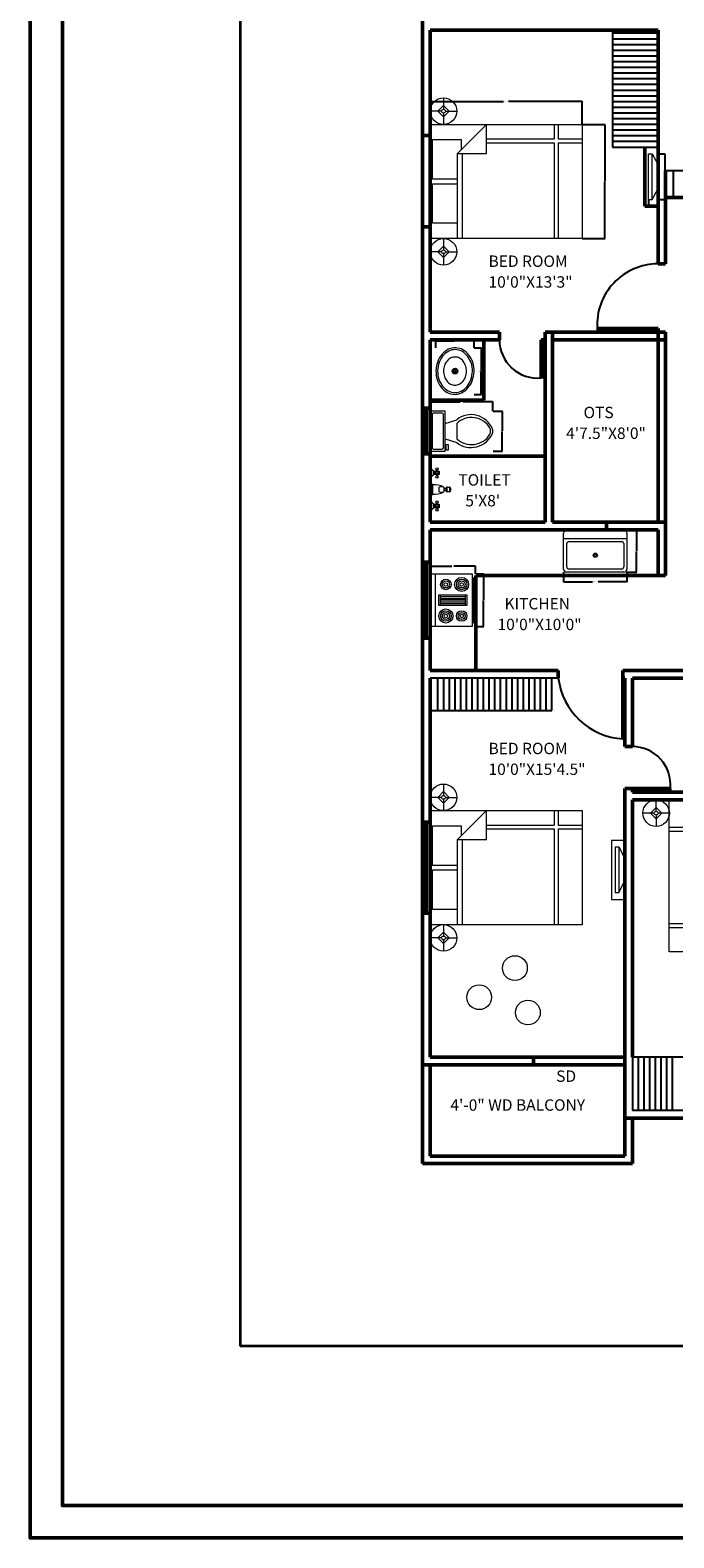
# Model space of a CAD drawing. Units: inches. Extents: x 1493 to 2377, y 814 to 2191.
# Tile 1 of 4: x 1493 to 1832, y 814 to 1607. Entities that reach past the tile are written whole.
import ezdxf

# ---------------------------------------------------------------- set-up
doc = ezdxf.new("R2010")
doc.units = ezdxf.units.IN
for name, color, linetype, lineweight in [('A-ANNO-DIMS', 2, 'Continuous', 18), ('A-ANNO-TTLB', 7, 'Continuous', 35), ('A-AREA-IDEN', 7, 'Continuous', 18), ('A-DOOR', 4, 'Continuous', 25), ('A-EQPM', 9, 'Continuous', 18), ('A-FLOR-FIXT', 8, 'Continuous', 18), ('A-FURN', 8, 'Continuous', 18), ('A-GLAZ', 4, 'Continuous', 25), ('A-WALL', 7, 'Continuous', 50)]:
    doc.layers.add(name, color=color, linetype=linetype, lineweight=lineweight)
doc.styles.get("Standard").update_dxf_attribs({"font": 'arial.ttf'})
doc.dimstyles.get("Standard").update_dxf_attribs({"dimtxt": 0.18, "dimasz": 0.18, "dimexe": 0.18, "dimexo": 0.0625, "dimgap": 0.09, "dimtad": 0, "dimtih": 1, "dimtoh": 1, "dimdec": 4, "dimzin": 0, "dimdsep": 46, "dimtxsty": 'Standard', "dimcen": 0.09, "dimadec": 0, "dimazin": 0, "dimtfac": 1, "dimtdec": 4, "dimtofl": 0, "dimtmove": 0, "dimatfit": 3, "dimfxl": 1, "dimtolj": 1, "dimtzin": 0, "dimarcsym": 0})

# ---------------------------------------------------------------- blocks, each defined once
blk = doc.blocks.new('Sink - Oval top')
for p, q in [((-1, 0), (1, 0)), ((0, 1), (0, -1))]:
    blk.add_line(p, q)
for points in [[(-12.23, 0.39, 0.117634), (-11.46, -3.36, 0.104469), (-8.88, -6.8, 0.090016), (-5.08, -9.07, 0.08192), (-0.32, -10.02, 0.08192), (4.49, -9.38, 0.090016), (8.42, -7.36, 0.104469), (11.22, -4.09, 0.117634), (12.23, -0.39, 0.117634), (11.46, 3.36, 0.104469), (8.88, 6.8, 0.090016), (5.08, 9.07, 0.08192), (0.32, 10.02, 0.08192), (-4.49, 9.38, 0.090016), (-8.42, 7.36, 0.104469), (-11.22, 4.09, 0.117634)], [(-11.29, 0.16, 0.118622), (-10.52, -3.25, 0.104678), (-8.07, -6.36, 0.089562), (-4.54, -8.37, 0.081185), (-0.13, -9.15, 0.081185), (4.3, -8.49, 0.089562), (7.89, -6.58, 0.104678), (10.42, -3.55, 0.118622), (11.29, -0.16, 0.118622), (10.52, 3.25, 0.104678), (8.07, 6.36, 0.089562), (4.54, 8.37, 0.081185), (0.13, 9.15, 0.081185), (-4.3, 8.49, 0.089562), (-7.89, 6.58, 0.104678), (-10.42, 3.55, 0.118622)], [(-7.42, 0.08, 0.118283), (-6.91, -2.17, 0.104607), (-5.29, -4.21, 0.089718), (-2.97, -5.53, 0.081436), (-0.07, -6.04, 0.081436), (2.84, -5.59, 0.089718), (5.2, -4.33, 0.104607), (6.86, -2.32, 0.118283), (7.42, -0.08, 0.118283), (6.91, 2.17, 0.104607), (5.29, 4.21, 0.089718), (2.97, 5.53, 0.081436), (0.07, 6.04, 0.081436), (-2.84, 5.59, 0.089718), (-5.2, 4.33, 0.104607), (-6.86, 2.32, 0.118283)]]:
    blk.add_lwpolyline(points, format="xyb", close=True)
for radius in [1.5, 1]:
    blk.add_circle((0, 0), radius)
blk = doc.blocks.new('Lamp - Table')
for p, q in [((-1, 0), (-7, 0)), ((0, 3), (-3, 0)), ((-3, 0), (0, -3)), ((0, 7), (0, 1)), ((3, 0), (0, 3)), ((0, -3), (3, 0)), ((1, 0), (7, 0)), ((0, -1), (0, -7))]:
    blk.add_line(p, q)
for radius in [7, 1]:
    blk.add_circle((0, 0), radius)
blk = doc.blocks.new('Bed - Queen')
for p, q in [((0, -80), (0, 0)), ((0, 0), (60, 0)), ((60, 0), (60, -80)), ((8, -1.2), (28.8, -1.2)), ((8, -14.4), (8, -1.2)), ((28.8, -1.2), (28.8, -14.4)), ((31.2, -1.2), (52, -1.2)), ((31.2, -14.4), (31.2, -1.2)), ((52, -1.2), (52, -16.4)), ((0, -14.4), (44.8, -14.4)), ((60, -29.6), (44.8, -14.4)), ((44.8, -14.4), (44.8, -29.6)), ((44.8, -16.8), (0, -16.8)), ((52, -16.4), (46.8, -16.4)), ((44.8, -29.6), (60, -29.6)), ((50.4, -29.6), (50.4, -65.35)), ((52.4, -29.6), (52.4, -65.35)), ((50.4, -65.35), (0, -65.35)), ((50.4, -67.35), (0, -67.35)), ((50.4, -67.35), (50.4, -80)), ((60, -65.35), (52.4, -65.35)), ((60, -67.35), (52.4, -67.35)), ((52.4, -67.35), (52.4, -80)), ((60, -80), (0, -80))]:
    blk.add_line(p, q)
blk = doc.blocks.new('Toilet - top')
for p, q in [((9.5, -6), (9.5, -2)), ((-10, -8.5), (-8, -8.5)), ((-10, -9.5), (-10, -8.5)), ((-7, -9.5), (-10, -9.5)), ((-8, -8.5), (-8, -8)), ((-7, -8), (-7, -9.5)), ((-4, -8), (-6, -14)), ((4, -14), (-4, -14)), ((4, -8), (6, -14))]:
    blk.add_line(p, q)
blk.add_lwpolyline([(10.5, -8), (10.5, 0), (-10.5, 0), (-10.5, -8)], close=True)
for points in [[(-9.5, -2), (-9.5, -6)], [(8.5, -1), (-8.5, -1)], [(-8.5, -7), (8.5, -7)]]:
    blk.add_lwpolyline(points)
for centre, radius, start, end in [((-8.62, -1.88), 0.884, 81.8699, 188.1301), ((-8.62, -6.12), 0.884, 171.8699, 278.1301), ((8.62, -1.88), 0.884, 351.8699, 98.1301), ((8.62, -6.12), 0.884, 261.8699, 8.1301), ((3.52, -21.58), 12.17, 141.46911, 247.97143), ((4.2, -21.82), 11.33, 136.36773, 238.94682), ((-3.52, -21.58), 12.17, 292.02843, 38.53071), ((-4.2, -21.82), 11.33, 301.05301, 43.63209), ((0, -27.88), 4, 245.73182, 294.26817), ((0, -29), 4, 254.86053, 285.13947)]:
    blk.add_arc(centre, radius, start, end)
blk = doc.blocks.new('Faucet - Bathroom front')
for p, q in [((-0.5, 4.25), (0.5, 4.25)), ((0.5, 3.75), (-0.5, 3.75)), ((-0.25, 3), (-0.25, 3.5)), ((0.25, 3.5), (0.25, 3)), ((-5, 0), (-2.25, 0)), ((-4.5087, 0.25), (-2.7408, 0.25)), ((-4, 1.625), (-4.25, 1.625)), ((-4, 1.375), (-4.25, 1.375)), ((-3.1442, 0.75), (-4.0979, 0.75)), ((-3.25, 1.625), (-3, 1.625)), ((-3.25, 1.375), (-3, 1.375)), ((-1.5, 0), (1.5, 0)), ((-1, 0.5), (1, 0.5)), ((-0.5, 3), (0.5, 3)), ((0.5, 2), (-0.5, 2)), ((2.25, 0), (5, 0)), ((2.7413, 0.25), (4.5092, 0.25)), ((3.25, 1.625), (3, 1.625)), ((3.25, 1.375), (3, 1.375)), ((4.1058, 0.75), (3.1521, 0.75)), ((4, 1.625), (4.25, 1.625)), ((4, 1.375), (4.25, 1.375))]:
    blk.add_line(p, q)
for points in [[(-0.5, 3.75), (-0.5, 4.25)], [(-0.25, 4.5), (0.25, 4.5)], [(0.25, 3.5), (-0.25, 3.5)], [(0.5, 4.25), (0.5, 3.75)]]:
    blk.add_lwpolyline(points)
for points in [[(-4, 1), (-4, 2), (-3.25, 2), (-3.25, 1)], [(3.25, 1), (3.25, 2), (4, 2), (4, 1)]]:
    blk.add_lwpolyline(points, close=True)
for centre in [(-4.5, 1.5), (-3.625, 1.5), (-2.75, 1.5), (2.75, 1.5), (3.625, 1.5), (4.5, 1.5)]:
    blk.add_circle(centre, 0.2795)
for centre, radius, start, end in [((-0.2575, 4.2575), 0.2426, 88.22243, 181.7776), ((-0.2575, 3.7425), 0.2426, 178.2224, 271.7776), ((0.2575, 4.2575), 0.2426, 358.2224, 91.77757), ((0.2575, 3.7425), 0.2426, 268.2224, 1.777565), ((-5.375, 1.375), 1.4252, 285.2551, 344.7449), ((-1.875, 1.375), 1.4252, 195.2551, 254.7449), ((-0.7962, -0.2038), 0.7327, 106.1502, 163.8498), ((3, 1), 4.0311, 150.2551, 187.125), ((0.6413, 2.5), 1.246, 156.3417, 203.6583), ((-3, 1), 4.0311, 352.875, 29.74488), ((-0.6413, 2.5), 1.246, 336.3417, 23.65835), ((0.7962, -0.2038), 0.7327, 16.1502, 73.84979), ((1.875, 1.375), 1.4252, 285.2551, 344.7449), ((5.375, 1.375), 1.4252, 195.2551, 254.7449)]:
    blk.add_arc(centre, radius, start, end)
blk = doc.blocks.new('Range-Oven - 30 in top')
for p, q in [((0, -3), (30, -3)), ((12, -6), (18, -6)), ((13, -20), (13, -6)), ((14, -6), (14, -20)), ((15, -20), (15, -6)), ((16, -6), (16, -20)), ((17, -20), (17, -6)), ((6, -24), (6, -25)), ((8, -25), (8, -24)), ((18, -20), (12, -20)), ((22, -25), (22, -24)), ((24, -24), (24, -25))]:
    blk.add_line(p, q)
for points in [[(0, -24), (0, 0), (30, 0), (30, -24)], [(12, -21), (12, -5), (18, -5), (18, -21)], [(2, -26), (2, -25), (28, -25), (28, -26)]]:
    blk.add_lwpolyline(points, close=True)
for centre, radius in [((6, -9), 4), ((6, -9), 3), ((6, -9), 2), ((6, -9), 1), ((24, -9), 3), ((24, -9), 2), ((24, -9), 1), ((6, -18), 3), ((6, -18), 2), ((6, -18), 1), ((24, -18), 4), ((24, -18), 3), ((24, -18), 2), ((24, -18), 1)]:
    blk.add_circle(centre, radius)
blk = doc.blocks.new('Sink-single - 30 in top')
blk.add_line((-15, -3.999996), (15, -3.999996))
for points in [[(-13.5, 0), (13.5, 0)], [(-15, -18.499996), (-15, -1.5)], [(-13.5, -17.499996), (-13.5, -6.499996)], [(-12.5, -5.499996), (12.5, -5.499996)], [(13.5, -6.499996), (13.5, -17.499996)], [(15, -1.5), (15, -18.499996)], [(13.5, -19.999996), (-13.5, -19.999996)], [(12.5, -18.499996), (-12.5, -18.499996)]]:
    blk.add_lwpolyline(points)
for radius in [1, 0.5]:
    blk.add_circle((0, -11.999996), radius)
for centre, radius, start, end in [((-13.5, -1.5), 1.5, 90, 180), ((-12.5, -6.499996), 1, 90, 180), ((12.5, -6.499996), 1, 0, 90), ((13.5, -1.5), 1.5, 0, 90), ((-13.5, -18.499996), 1.5, 180, 270), ((-12.5, -17.499996), 1, 180, 270), ((12.5, -17.499996), 1, 270, 0), ((13.5, -18.499996), 1.5, 270, 0)]:
    blk.add_arc(centre, radius, start, end)
blk = doc.blocks.new('AC-SPLIT-UNIT')
for p, q in [((-2, 27.5), (-2, -3.65)), ((-2, 27.5), (5, 27.5)), ((0, 24), (2, 24)), ((0, 24), (0, 0)), ((2, 24), (2, 0)), ((2, 24), (5, 18.22)), ((2, 0), (5, 5.78)), ((-2, -3.65), (5, -3.65)), ((0, 0), (2, 0))]:
    blk.add_line(p, q)
blk = doc.blocks.new('AC-INDOOR-UNIT')
for p, q in [((0, 0), (0, 24)), ((0, 24), (2, 24)), ((2, 0), (2, 24)), ((2, 24), (5, 18.22)), ((2, 0), (5, 5.78)), ((0, 0), (2, 0))]:
    blk.add_line(p, q)
blk = doc.blocks.new('*D12')
at = {"layer": 'A-ANNO-DIMS', "color": 0, "lineweight": -2, "transparency": 16777216}
for p, q in [((1703.83, 1557.8), (1703.83, 1569.92)), ((1704.01, 1569.74), (1742.53, 1569.74)), ((1783.65, 1569.74), (1745.14, 1569.74)), ((1783.83, 1557.8), (1783.83, 1569.92))]:
    blk.add_line(p, q, dxfattribs=at)
at = {"layer": 'A-ANNO-DIMS', "color": 0, "transparency": 16777216}
for points in [[(1704.01, 1569.77), (1704.01, 1569.71), (1703.83, 1569.74)], [(1783.65, 1569.77), (1783.65, 1569.71), (1783.83, 1569.74)]]:
    blk.add_solid(points, dxfattribs=at)
at = {"layer": 'Defpoints', "color": 0, "transparency": 16777216}
for p in [(1703.83, 1569.74), (1703.83, 1557.74), (1783.83, 1557.74)]:
    blk.add_point(p, dxfattribs=at)
at = {"layer": 'A-ANNO-DIMS', "color": 0, "transparency": 16777216, "insert": (1743.83, 1569.74), "char_height": 0.18, "attachment_point": 5}
blk.add_mtext('\\A1;QUEEN BED 80 TYP.', dxfattribs=at)
blk = doc.blocks.new('*D13')
at = {"layer": 'A-ANNO-DIMS', "color": 0, "lineweight": -2, "transparency": 16777216}
for p, q in [((1783.9, 1557.74), (1796.01, 1557.74)), ((1795.83, 1557.56), (1795.83, 1527.92)), ((1795.83, 1497.92), (1795.83, 1527.56)), ((1783.9, 1497.74), (1796.01, 1497.74))]:
    blk.add_line(p, q, dxfattribs=at)
at = {"layer": 'A-ANNO-DIMS', "color": 0, "transparency": 16777216}
for points in [[(1795.8, 1557.56), (1795.86, 1557.56), (1795.83, 1557.74)], [(1795.8, 1497.92), (1795.86, 1497.92), (1795.83, 1497.74)]]:
    blk.add_solid(points, dxfattribs=at)
at = {"layer": 'Defpoints', "color": 0, "transparency": 16777216}
for p in [(1783.83, 1557.74), (1795.83, 1557.74), (1783.83, 1497.74)]:
    blk.add_point(p, dxfattribs=at)
at = {"layer": 'A-ANNO-DIMS', "color": 0, "transparency": 16777216, "insert": (1795.83, 1527.74), "char_height": 0.18, "attachment_point": 5}
blk.add_mtext('\\A1;60 TYP.', dxfattribs=at)
blk = doc.blocks.new('*D16')
at = {"layer": 'A-ANNO-DIMS', "color": 0, "lineweight": -2, "transparency": 16777216}
for p, q in [((1727.07, 1440.21), (1730.87, 1440.21)), ((1730.69, 1440.03), (1730.69, 1428.12)), ((1730.69, 1415.84), (1730.69, 1427.75)), ((1727.07, 1415.66), (1730.87, 1415.66))]:
    blk.add_line(p, q, dxfattribs=at)
at = {"layer": 'A-ANNO-DIMS', "color": 0, "transparency": 16777216}
for points in [[(1730.66, 1440.03), (1730.72, 1440.03), (1730.69, 1440.21)], [(1730.66, 1415.84), (1730.72, 1415.84), (1730.69, 1415.66)]]:
    blk.add_solid(points, dxfattribs=at)
at = {"layer": 'Defpoints', "color": 0, "transparency": 16777216}
for p in [(1727.01, 1440.21), (1730.69, 1440.21), (1727.01, 1415.66)]:
    blk.add_point(p, dxfattribs=at)
at = {"layer": 'A-ANNO-DIMS', "color": 0, "transparency": 16777216, "insert": (1730.69, 1427.94), "char_height": 0.18, "attachment_point": 5}
blk.add_mtext('\\A1;WASH BASIN 25 TYP.', dxfattribs=at)
blk = doc.blocks.new('*D17')
at = {"layer": 'A-ANNO-DIMS', "color": 0, "lineweight": -2, "transparency": 16777216}
for p, q in [((1706.88, 1440.27), (1706.88, 1444.07)), ((1727.01, 1440.27), (1727.01, 1444.07)), ((1707.06, 1443.89), (1716.41, 1443.89)), ((1726.83, 1443.89), (1717.47, 1443.89))]:
    blk.add_line(p, q, dxfattribs=at)
at = {"layer": 'A-ANNO-DIMS', "color": 0, "transparency": 16777216}
for points in [[(1707.06, 1443.92), (1707.06, 1443.86), (1706.88, 1443.89)], [(1726.83, 1443.92), (1726.83, 1443.86), (1727.01, 1443.89)]]:
    blk.add_solid(points, dxfattribs=at)
at = {"layer": 'Defpoints', "color": 0, "transparency": 16777216}
for p in [(1706.88, 1443.89), (1706.88, 1440.21), (1727.01, 1440.21)]:
    blk.add_point(p, dxfattribs=at)
at = {"layer": 'A-ANNO-DIMS', "color": 0, "transparency": 16777216, "insert": (1716.94, 1443.89), "char_height": 0.18, "attachment_point": 5}
blk.add_mtext('\\A1;20 TYP.', dxfattribs=at)
blk = doc.blocks.new('*D22')
at = {"layer": 'A-ANNO-DIMS', "color": 0, "lineweight": -2, "transparency": 16777216}
for p, q in [((1703.83, 1406.93), (1703.83, 1412)), ((1704.01, 1411.82), (1719.58, 1411.82)), ((1736.7, 1411.82), (1721.13, 1411.82)), ((1736.88, 1406.93), (1736.88, 1412))]:
    blk.add_line(p, q, dxfattribs=at)
at = {"layer": 'A-ANNO-DIMS', "color": 0, "transparency": 16777216}
for points in [[(1704.01, 1411.85), (1704.01, 1411.79), (1703.83, 1411.82)], [(1736.7, 1411.85), (1736.7, 1411.79), (1736.88, 1411.82)]]:
    blk.add_solid(points, dxfattribs=at)
at = {"layer": 'Defpoints', "color": 0, "transparency": 16777216}
for p in [(1703.83, 1411.82), (1703.83, 1406.87), (1736.88, 1406.87)]:
    blk.add_point(p, dxfattribs=at)
at = {"layer": 'A-ANNO-DIMS', "color": 0, "transparency": 16777216, "insert": (1720.36, 1411.82), "char_height": 0.18, "attachment_point": 5}
blk.add_mtext('\\A1;WC 33 TYP.', dxfattribs=at)
blk = doc.blocks.new('*D23')
at = {"layer": 'A-ANNO-DIMS', "color": 0, "lineweight": -2, "transparency": 16777216}
for p, q in [((1736.94, 1406.87), (1742.02, 1406.87)), ((1741.84, 1406.69), (1741.84, 1396.55)), ((1741.84, 1386.05), (1741.84, 1396.19)), ((1736.94, 1385.87), (1742.02, 1385.87))]:
    blk.add_line(p, q, dxfattribs=at)
at = {"layer": 'A-ANNO-DIMS', "color": 0, "transparency": 16777216}
for points in [[(1741.81, 1406.69), (1741.87, 1406.69), (1741.84, 1406.87)], [(1741.81, 1386.05), (1741.87, 1386.05), (1741.84, 1385.87)]]:
    blk.add_solid(points, dxfattribs=at)
at = {"layer": 'Defpoints', "color": 0, "transparency": 16777216}
for p in [(1736.88, 1406.87), (1741.84, 1406.87), (1736.88, 1385.87)]:
    blk.add_point(p, dxfattribs=at)
at = {"layer": 'A-ANNO-DIMS', "color": 0, "transparency": 16777216, "insert": (1741.84, 1396.37), "char_height": 0.18, "attachment_point": 5}
blk.add_mtext('\\A1;21 TYP.', dxfattribs=at)
blk = doc.blocks.new('*D26')
at = {"layer": 'A-ANNO-DIMS', "color": 0, "lineweight": -2, "transparency": 16777216}
for p, q in [((1727.88, 1321.2), (1732.14, 1321.2)), ((1731.96, 1321.02), (1731.96, 1307.55)), ((1731.96, 1293.71), (1731.96, 1307.18)), ((1727.88, 1293.53), (1732.14, 1293.53))]:
    blk.add_line(p, q, dxfattribs=at)
at = {"layer": 'A-ANNO-DIMS', "color": 0, "transparency": 16777216}
for points in [[(1731.93, 1321.02), (1731.99, 1321.02), (1731.96, 1321.2)], [(1731.93, 1293.71), (1731.99, 1293.71), (1731.96, 1293.53)]]:
    blk.add_solid(points, dxfattribs=at)
at = {"layer": 'Defpoints', "color": 0, "transparency": 16777216}
for p in [(1727.81, 1321.2), (1731.96, 1321.2), (1727.81, 1293.53)]:
    blk.add_point(p, dxfattribs=at)
at = {"layer": 'A-ANNO-DIMS', "color": 0, "transparency": 16777216, "insert": (1731.96, 1307.37), "char_height": 0.18, "attachment_point": 5}
blk.add_mtext('\\A1;RANGE/OVEN 28 TYP.', dxfattribs=at)
blk = doc.blocks.new('*D27')
at = {"layer": 'A-ANNO-DIMS', "color": 0, "lineweight": -2, "transparency": 16777216}
for p, q in [((1703.83, 1321.26), (1703.83, 1325.53)), ((1704.01, 1325.35), (1715.29, 1325.35)), ((1727.63, 1325.35), (1716.35, 1325.35)), ((1727.81, 1321.26), (1727.81, 1325.53))]:
    blk.add_line(p, q, dxfattribs=at)
at = {"layer": 'A-ANNO-DIMS', "color": 0, "transparency": 16777216}
for points in [[(1704.01, 1325.38), (1704.01, 1325.32), (1703.83, 1325.35)], [(1727.63, 1325.38), (1727.63, 1325.32), (1727.81, 1325.35)]]:
    blk.add_solid(points, dxfattribs=at)
at = {"layer": 'Defpoints', "color": 0, "transparency": 16777216}
for p in [(1703.83, 1325.35), (1703.83, 1321.2), (1727.81, 1321.2)]:
    blk.add_point(p, dxfattribs=at)
at = {"layer": 'A-ANNO-DIMS', "color": 0, "transparency": 16777216, "insert": (1715.82, 1325.35), "char_height": 0.18, "attachment_point": 5}
blk.add_mtext('\\A1;24 TYP.', dxfattribs=at)
blk = doc.blocks.new('*D28')
at = {"layer": 'A-ANNO-DIMS', "color": 0, "lineweight": -2, "transparency": 16777216}
for p, q in [((1774.12, 1322.06), (1774.12, 1316.94)), ((1774.3, 1317.12), (1789.37, 1317.12)), ((1807.31, 1317.12), (1792.25, 1317.12)), ((1807.49, 1322.06), (1807.49, 1316.94))]:
    blk.add_line(p, q, dxfattribs=at)
at = {"layer": 'A-ANNO-DIMS', "color": 0, "transparency": 16777216}
for points in [[(1774.3, 1317.15), (1774.3, 1317.09), (1774.12, 1317.12)], [(1807.31, 1317.15), (1807.31, 1317.09), (1807.49, 1317.12)]]:
    blk.add_solid(points, dxfattribs=at)
at = {"layer": 'Defpoints', "color": 0, "transparency": 16777216}
for p in [(1774.12, 1322.12), (1807.49, 1322.12), (1807.49, 1317.12)]:
    blk.add_point(p, dxfattribs=at)
at = {"layer": 'A-ANNO-DIMS', "color": 0, "transparency": 16777216, "insert": (1790.81, 1317.12), "char_height": 0.18, "attachment_point": 5}
blk.add_mtext('\\A1;KITCHEN SINK 33 TYP.', dxfattribs=at)
blk = doc.blocks.new('*D29')
at = {"layer": 'A-ANNO-DIMS', "color": 0, "lineweight": -2, "transparency": 16777216}
for p, q in [((1807.55, 1344.37), (1812.68, 1344.37)), ((1812.5, 1344.19), (1812.5, 1333.43)), ((1812.5, 1322.3), (1812.5, 1333.06)), ((1807.55, 1322.12), (1812.68, 1322.12))]:
    blk.add_line(p, q, dxfattribs=at)
at = {"layer": 'A-ANNO-DIMS', "color": 0, "transparency": 16777216}
for points in [[(1812.47, 1344.19), (1812.53, 1344.19), (1812.5, 1344.37)], [(1812.47, 1322.3), (1812.53, 1322.3), (1812.5, 1322.12)]]:
    blk.add_solid(points, dxfattribs=at)
at = {"layer": 'Defpoints', "color": 0, "transparency": 16777216}
for p in [(1807.49, 1344.37), (1812.5, 1344.37), (1807.49, 1322.12)]:
    blk.add_point(p, dxfattribs=at)
at = {"layer": 'A-ANNO-DIMS', "color": 0, "transparency": 16777216, "insert": (1812.5, 1333.24), "char_height": 0.18, "attachment_point": 5}
blk.add_mtext('\\A1;22 TYP.', dxfattribs=at)
blk = doc.blocks.new('*D40')
at = {"layer": 'A-ANNO-DIMS', "color": 0, "lineweight": -2, "transparency": 16777216}
for p, q in [((1823.9, 1542.21), (1827.61, 1542.21)), ((1827.43, 1542.03), (1827.43, 1530.4)), ((1827.43, 1518.39), (1827.43, 1530.03)), ((1823.9, 1518.21), (1827.61, 1518.21))]:
    blk.add_line(p, q, dxfattribs=at)
at = {"layer": 'A-ANNO-DIMS', "color": 0, "transparency": 16777216}
for points in [[(1827.4, 1542.03), (1827.46, 1542.03), (1827.43, 1542.21)], [(1827.4, 1518.39), (1827.46, 1518.39), (1827.43, 1518.21)]]:
    blk.add_solid(points, dxfattribs=at)
at = {"layer": 'Defpoints', "color": 0, "transparency": 16777216}
for p in [(1823.83, 1542.21), (1827.43, 1542.21), (1823.83, 1518.21)]:
    blk.add_point(p, dxfattribs=at)
at = {"layer": 'A-ANNO-DIMS', "color": 0, "transparency": 16777216, "insert": (1827.43, 1530.21), "char_height": 0.18, "attachment_point": 5}
blk.add_mtext('\\A1;AC INDOOR UNIT 24 TYP.', dxfattribs=at)
blk = doc.blocks.new('*D41')
at = {"layer": 'A-ANNO-DIMS', "color": 0, "lineweight": -2, "transparency": 16777216}
for p, q in [((1818.83, 1518.15), (1818.83, 1514.43)), ((1823.83, 1518.15), (1823.83, 1514.43)), ((1819.01, 1514.61), (1820.87, 1514.61)), ((1823.65, 1514.61), (1821.79, 1514.61))]:
    blk.add_line(p, q, dxfattribs=at)
at = {"layer": 'A-ANNO-DIMS', "color": 0, "transparency": 16777216}
for points in [[(1819.01, 1514.64), (1819.01, 1514.58), (1818.83, 1514.61)], [(1823.65, 1514.64), (1823.65, 1514.58), (1823.83, 1514.61)]]:
    blk.add_solid(points, dxfattribs=at)
at = {"layer": 'Defpoints', "color": 0, "transparency": 16777216}
for p in [(1818.83, 1518.21), (1823.83, 1518.21), (1823.83, 1514.61)]:
    blk.add_point(p, dxfattribs=at)
at = {"layer": 'A-ANNO-DIMS', "color": 0, "transparency": 16777216, "insert": (1821.33, 1514.61), "char_height": 0.18, "attachment_point": 5}
blk.add_mtext('\\A1;5 TYP.', dxfattribs=at)

msp = doc.modelspace()

# ---------------------------------------------------------------- linework, layer by layer
at = {"layer": 'A-ANNO-TTLB'}
for p in [(1603.83, 2093.87), (2271.83, 914.87)]:
    msp.add_line(p, (1603.83, 914.87), dxfattribs=at)
at = {"layer": 'A-DOOR'}
for p, q in [((1791.83, 1450.37), (1791.83, 1449.37)), ((1763.33, 1424.37), (1762.33, 1424.37)), ((1806.33, 1266.37), (1806.33, 1234.37)), ((1830.33, 1208.37), (1830.33, 1207.37))]:
    msp.add_line(p, q, dxfattribs=at)
for centre, radius, start, end in [((1823.83, 1452.31), 32.06, 90, 183.47141), ((1760.42, 1444.37), 20.09, 180, 275.45262), ((1807.62, 1270.86), 36.57, 187.0603, 266.41111), ((1810.33, 1210.28), 20.09, 354.54738, 90)]:
    msp.add_arc(centre, radius, start, end, dxfattribs=at)
at = {"layer": 'A-FURN'}
for centre in [(1748.48, 1113.75), (1729.66, 1098.44), (1755.31, 1090.4)]:
    msp.add_circle(centre, 6.53, dxfattribs=at)
at = {"layer": 'A-GLAZ'}
for p, q in [((1799.83, 1607.37), (1799.83, 1545.87)), ((1799.83, 1605.87), (1823.83, 1605.87)), ((1799.83, 1602.87), (1823.83, 1602.87)), ((1799.83, 1599.87), (1823.83, 1599.87)), ((1799.83, 1596.87), (1823.83, 1596.87)), ((1799.83, 1593.87), (1823.83, 1593.87)), ((1799.83, 1590.87), (1823.83, 1590.87)), ((1799.83, 1587.87), (1823.83, 1587.87)), ((1799.83, 1584.87), (1823.83, 1584.87)), ((1799.83, 1581.87), (1823.83, 1581.87)), ((1799.83, 1578.87), (1823.83, 1578.87)), ((1799.83, 1575.87), (1823.83, 1575.87)), ((1799.83, 1572.87), (1823.83, 1572.87)), ((1799.83, 1569.87), (1823.83, 1569.87)), ((1799.83, 1566.87), (1823.83, 1566.87)), ((1799.83, 1563.87), (1823.83, 1563.87)), ((1799.83, 1560.87), (1823.83, 1560.87)), ((1799.83, 1557.87), (1823.83, 1557.87)), ((1799.83, 1554.87), (1823.83, 1554.87)), ((1799.83, 1551.87), (1823.83, 1551.87)), ((1799.83, 1548.87), (1823.83, 1548.87)), ((1799.83, 1545.87), (1823.83, 1545.87)), ((1816.83, 1545.87), (1823.83, 1545.87)), ((1897.83, 1533.37), (1827.83, 1533.37)), ((1831.83, 1533.37), (1831.83, 1519.37)), ((1771.33, 1266.37), (1703.83, 1266.37)), ((1707.97, 1249.35), (1707.97, 1266.37)), ((1710.97, 1249.35), (1710.97, 1266.37)), ((1713.97, 1249.35), (1713.97, 1266.37)), ((1716.97, 1249.35), (1716.97, 1266.37)), ((1719.97, 1249.35), (1719.97, 1266.37)), ((1722.97, 1249.35), (1722.97, 1266.37)), ((1725.97, 1249.35), (1725.97, 1266.37)), ((1728.97, 1249.35), (1728.97, 1266.37)), ((1731.97, 1249.35), (1731.97, 1266.37)), ((1734.97, 1249.35), (1734.97, 1266.37)), ((1737.97, 1249.35), (1737.97, 1266.37)), ((1740.97, 1249.35), (1740.97, 1266.37)), ((1743.97, 1249.35), (1743.97, 1266.37)), ((1746.97, 1249.35), (1746.97, 1266.37)), ((1749.97, 1249.35), (1749.97, 1266.37)), ((1752.97, 1249.35), (1752.97, 1266.37)), ((1755.97, 1249.35), (1755.97, 1266.37)), ((1758.97, 1249.35), (1758.97, 1266.37)), ((1761.97, 1249.35), (1761.97, 1266.37)), ((1764.97, 1249.35), (1764.97, 1266.37)), ((1767.97, 1249.35), (1767.97, 1266.37)), ((1703.83, 1249.35), (1767.97, 1249.35)), ((1855.33, 1066.87), (1810.33, 1066.87)), ((1810.33, 1066.87), (1810.33, 1038.87)), ((1813.33, 1066.87), (1813.33, 1038.87)), ((1816.33, 1066.87), (1816.33, 1038.87)), ((1819.33, 1066.87), (1819.33, 1038.87)), ((1822.33, 1066.87), (1822.33, 1038.87)), ((1825.33, 1066.87), (1825.33, 1038.87)), ((1828.33, 1066.87), (1828.33, 1038.87)), ((1831.33, 1066.87), (1831.33, 1038.87)), ((1858.33, 1038.87), (1810.33, 1038.87))]:
    msp.add_line(p, q, dxfattribs=at)
at = {"layer": 'A-WALL'}
for p, q in [((1699.83, 1997.87), (1699.83, 1010.87)), ((1823.83, 1607.37), (1703.83, 1607.37)), ((1703.83, 1607.37), (1703.83, 1448.37)), ((1823.83, 1607.37), (1823.83, 1484.37)), ((1703.83, 1551.87), (1699.83, 1551.87)), ((1816.83, 1514.71), (1816.83, 1545.87)), ((1827.83, 1533.37), (1827.83, 1484.37)), ((1901.83, 1519.37), (1827.83, 1519.37)), ((1816.83, 1514.71), (1823.83, 1514.71)), ((1703.83, 1503.87), (1699.83, 1503.87)), ((1827.83, 1484.37), (1823.83, 1484.37)), ((1740.33, 1448.37), (1703.83, 1448.37)), ((1740.33, 1444.37), (1703.83, 1444.37)), ((1703.83, 1444.37), (1703.83, 1348.37)), ((1732.15, 1412.56), (1732.15, 1444.37)), ((1740.33, 1448.37), (1740.33, 1444.37)), ((1764.33, 1444.37), (1762.33, 1444.37)), ((1762.33, 1444.37), (1762.33, 1424.37)), ((1763.33, 1444.37), (1763.33, 1424.37)), ((1764.33, 1448.37), (1764.33, 1348.37)), ((1827.83, 1448.37), (1764.33, 1448.37)), ((1768.33, 1448.37), (1768.33, 1348.37)), ((1827.83, 1444.37), (1768.33, 1444.37)), ((1823.83, 1450.37), (1791.83, 1450.37)), ((1823.83, 1449.37), (1791.83, 1449.37)), ((1823.83, 1450.37), (1823.83, 1348.37)), ((1827.83, 1448.37), (1827.83, 1320.37)), ((1732.15, 1412.56), (1703.83, 1412.56)), ((1703.83, 1408.37), (1699.83, 1408.37)), ((1701.83, 1408.37), (1701.83, 1384.37)), ((1703.83, 1384.37), (1699.83, 1384.37)), ((1703.83, 1383.23), (1764.33, 1383.23)), ((1764.33, 1348.37), (1703.83, 1348.37)), ((1823.83, 1344.37), (1703.83, 1344.37)), ((1703.83, 1344.37), (1703.83, 1270.37)), ((1827.83, 1348.37), (1768.33, 1348.37)), ((1796.72, 1348.37), (1796.72, 1344.37)), ((1823.83, 1344.37), (1823.83, 1320.37)), ((1703.83, 1327.37), (1699.83, 1327.37)), ((1701.83, 1327.37), (1701.83, 1287.37)), ((1827.83, 1320.37), (1727.83, 1320.37)), ((1727.83, 1320.37), (1727.83, 1270.37)), ((1703.83, 1287.37), (1699.83, 1287.37)), ((1771.33, 1270.37), (1703.83, 1270.37)), ((1771.33, 1266.37), (1771.33, 1270.37)), ((1805.33, 1270.37), (1805.33, 1234.37)), ((1810.33, 1270.37), (1805.33, 1270.37)), ((1870.33, 1270.37), (1805.33, 1270.37)), ((1703.83, 1266.37), (1703.83, 1066.87)), ((1806.33, 1266.37), (1805.33, 1266.37)), ((1806.33, 1266.37), (1805.33, 1266.37)), ((1806.33, 1266.37), (1806.33, 1230.37)), ((1810.33, 1266.37), (1810.33, 1230.37)), ((1870.33, 1266.37), (1810.33, 1266.37)), ((1810.33, 1230.37), (1806.33, 1230.37)), ((1830.33, 1208.37), (1806.33, 1208.37)), ((1806.33, 1208.37), (1806.33, 1202.37)), ((1806.33, 1206.37), (1806.33, 1066.87)), ((1830.33, 1207.37), (1810.33, 1207.37)), ((1810.33, 1207.37), (1810.33, 1206.37)), ((1894.33, 1206.37), (1810.33, 1206.37)), ((1810.33, 1202.37), (1810.33, 1066.87)), ((1933.89, 1202.37), (1810.33, 1202.37)), ((1703.83, 1190.62), (1699.83, 1190.62)), ((1701.83, 1190.62), (1701.83, 1142.62)), ((1703.83, 1142.62), (1699.83, 1142.62)), ((1806.33, 1066.87), (1703.83, 1066.87)), ((1758.33, 1066.87), (1758.33, 1062.87)), ((1806.33, 1066.87), (1806.33, 1062.87)), ((1806.33, 1062.87), (1699.83, 1062.87)), ((1703.83, 1062.87), (1703.83, 1014.87)), ((1806.33, 1062.87), (1806.33, 1014.87)), ((1862.33, 1034.87), (1806.33, 1034.87)), ((1810.33, 1034.87), (1810.33, 1010.87)), ((1810.33, 1010.87), (1699.83, 1010.87)), ((1806.33, 1014.87), (1703.83, 1014.87))]:
    msp.add_line(p, q, dxfattribs=at)
for points in [[(1493.21, 2190.87), (2376.73, 2190.87), (2376.73, 813.94), (1493.21, 813.94)], [(1510.21, 2173.87), (2359.73, 2173.87), (2359.73, 830.94), (1510.21, 830.94)]]:
    msp.add_lwpolyline(points, close=True, dxfattribs=at)

# ---------------------------------------------------------------- block references
at = {"layer": 'A-EQPM'}
for name, p in [('AC-INDOOR-UNIT', (1818.83, 1518.21)), ('AC-SPLIT-UNIT', (1801.26, 1153.51))]:
    msp.add_blockref(name, p, dxfattribs=at)
at = {"layer": 'A-EQPM', "xscale": 0.9223664776301376, "yscale": 0.9223664776301376, "zscale": 0.9223664776301376, "rotation": 90}
msp.add_blockref('Range-Oven - 30 in top', (1703.83, 1293.53), dxfattribs=at)
at = {"layer": 'A-FLOR-FIXT', "rotation": 90}
for name, p in [('Sink - Oval top', (1716.94, 1427.94)), ('Toilet - top', (1703.83, 1396.37))]:
    msp.add_blockref(name, p, dxfattribs=at)
at = {"layer": 'A-FLOR-FIXT', "xscale": 2.398174673042902, "yscale": 2.398174673042902, "zscale": 2.398174673042902, "rotation": 270.0000081786288}
msp.add_blockref('Faucet - Bathroom front', (1703.83, 1365.65), dxfattribs=at)
at = {"layer": 'A-FLOR-FIXT', "xscale": 1.112314284845436, "yscale": 1.112314284845436, "zscale": 1.112314284845436}
msp.add_blockref('Sink-single - 30 in top', (1790.81, 1344.37), dxfattribs=at)
at = {"layer": 'A-FURN'}
for name, p in [('Lamp - Table', (1710.86, 1564.74)), ('Lamp - Table', (1710.86, 1490.75)), ('Lamp - Table', (1710.86, 1203.62)), ('Bed - Queen', (1829.79, 1202.37)), ('Lamp - Table', (1710.86, 1129.63))]:
    msp.add_blockref(name, p, dxfattribs=at)
for name, p, rotation in [('Bed - Queen', (1703.83, 1497.74), 90), ('Lamp - Table', (1822.81, 1195.33), 270), ('Bed - Queen', (1703.83, 1136.62), 90)]:
    msp.add_blockref(name, p, dxfattribs=dict(at, rotation=rotation))

# ---------------------------------------------------------------- texts
at = {"layer": 'A-AREA-IDEN'}
for s, p in [('BED ROOM', (1734.58, 1482.78)), ('10\'0"X13\'3"', (1734.58, 1471.85)), ('      OTS', (1773.63, 1403.17)), (' 4\'7.5"X8\'0"', (1773.63, 1392.25)), ('TOILET', (1718.7, 1367.67)), ("  5'X8'", (1718.7, 1356.75)), ('  KITCHEN', (1739.33, 1302.53)), ('10\'0"X10\'0"', (1739.33, 1291.61)), ('BED ROOM', (1734.58, 1226.35)), ('10\'0"X15\'4.5"', (1734.58, 1215.42)), ('      SD', (1759.21, 1053.9)), ('4\'-0" WD BALCONY', (1714.49, 1038.71))]:
    msp.add_text(s, height=6, dxfattribs=at).set_placement(p)

# ---------------------------------------------------------------- dimensions: what is measured, and where the dimension line sits
at = {"layer": 'A-ANNO-DIMS'}
for base, p1, p2, angle, text, picture, middle in [((1703.83, 1569.74), (1783.83, 1557.74), (1703.83, 1557.74), 180, 'QUEEN BED <> TYP.', '*D12', (1743.83, 1569.74)), ((1795.83, 1557.74), (1783.83, 1497.74), (1783.83, 1557.74), 90, '<> TYP.', '*D13', (1795.83, 1527.74)), ((1827.43, 1542.21), (1823.83, 1518.21), (1823.83, 1542.21), 90, 'AC INDOOR UNIT <> TYP.', '*D40', (1827.43, 1530.21)), ((1706.88, 1443.89), (1727.01, 1440.21), (1706.88, 1440.21), 180, '<> TYP.', '*D17', (1716.94, 1443.89)), ((1730.69, 1440.21), (1727.01, 1415.66), (1727.01, 1440.21), 90, 'WASH BASIN <> TYP.', '*D16', (1730.69, 1427.94)), ((1703.83, 1411.82), (1736.88, 1406.87), (1703.83, 1406.87), 180, 'WC <> TYP.', '*D22', (1720.36, 1411.82)), ((1741.84, 1406.87), (1736.88, 1385.87), (1736.88, 1406.87), 90, '<> TYP.', '*D23', (1741.84, 1396.37)), ((1812.5, 1344.37), (1807.49, 1322.12), (1807.49, 1344.37), 90, '<> TYP.', '*D29', (1812.5, 1333.24)), ((1703.83, 1325.35), (1727.81, 1321.2), (1703.83, 1321.2), 180, '<> TYP.', '*D27', (1715.82, 1325.35)), ((1731.96, 1321.2), (1727.81, 1293.53), (1727.81, 1321.2), 90, 'RANGE/OVEN <> TYP.', '*D26', (1731.96, 1307.37))]:
    dim = msp.add_linear_dim(base=base, p1=p1, p2=p2, angle=angle, text=text, dimstyle='Standard', override={"dimdec": 0, "dimlfac": 1, "dimrnd": 0, "dimzin": 0, "dimdsep": 46, "dimlunit": 2}, dxfattribs=at)
    dim.commit()
    dim.dimension.update_dxf_attribs({"geometry": picture, "text_midpoint": middle})
for base, p1, p2, text, picture, middle in [((1823.83, 1514.61), (1818.83, 1518.21), (1823.83, 1518.21), '<> TYP.', '*D41', (1821.33, 1514.61)), ((1807.49, 1317.12), (1774.12, 1322.12), (1807.49, 1322.12), 'KITCHEN SINK <> TYP.', '*D28', (1790.81, 1317.12))]:
    dim = msp.add_linear_dim(base=base, p1=p1, p2=p2, text=text, dimstyle='Standard', override={"dimdec": 0, "dimlfac": 1, "dimrnd": 0, "dimzin": 0, "dimdsep": 46, "dimlunit": 2}, dxfattribs=at)
    dim.commit()
    dim.dimension.update_dxf_attribs({"geometry": picture, "text_midpoint": middle})

doc.saveas('drawing.dxf')
